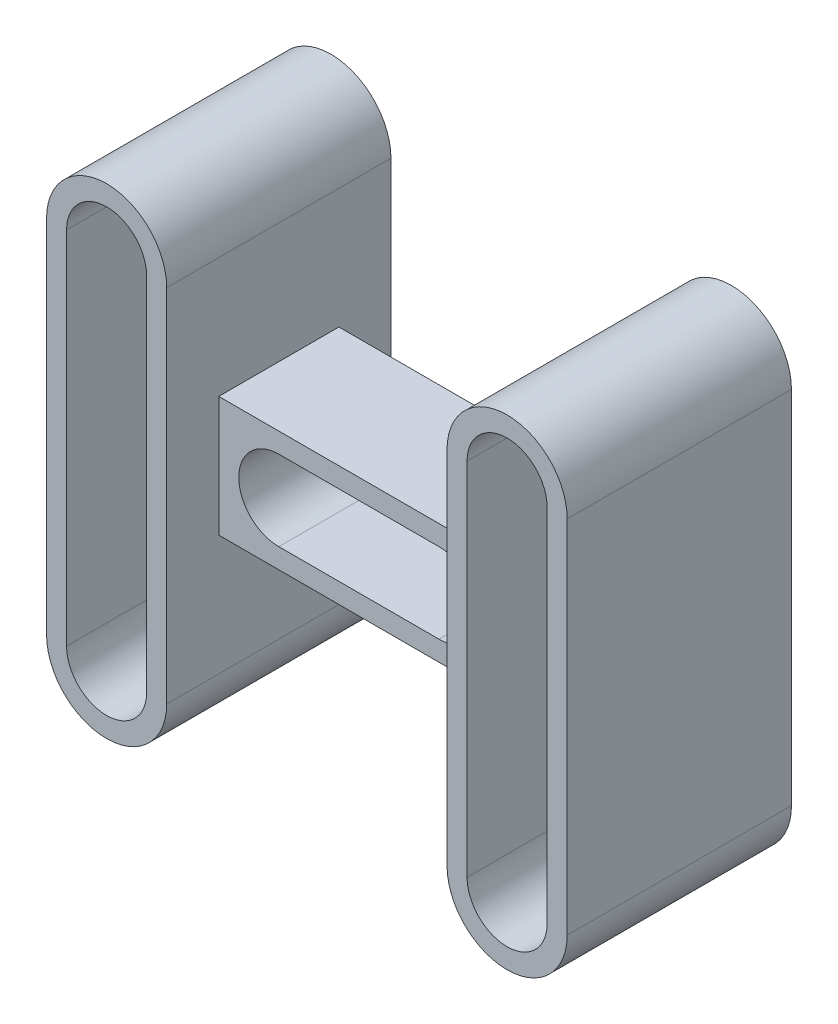
ISO-10303-21;
HEADER;
FILE_DESCRIPTION(('STEP AP214'),'2;1');
FILE_NAME('part.step','',(''),(''),'','','');
FILE_SCHEMA(('AUTOMOTIVE_DESIGN { 1 0 10303 214 1 1 1 1 }'));
ENDSEC;
DATA;
#1=APPLICATION_CONTEXT('core data for automotive mechanical design processes');
#2=APPLICATION_PROTOCOL_DEFINITION('international standard','automotive_design',2000,#1);
#3=PRODUCT_CONTEXT('',#1,'mechanical');
#4=PRODUCT('Part','Part','',(#3));
#5=PRODUCT_RELATED_PRODUCT_CATEGORY('part','',(#4));
#6=PRODUCT_DEFINITION_FORMATION('','',#4);
#7=PRODUCT_DEFINITION_CONTEXT('part definition',#1,'design');
#8=PRODUCT_DEFINITION('design','',#6,#7);
#9=PRODUCT_DEFINITION_SHAPE('','',#8);
#10=(LENGTH_UNIT() NAMED_UNIT(*) SI_UNIT(.MILLI.,.METRE.));
#11=(NAMED_UNIT(*) PLANE_ANGLE_UNIT() SI_UNIT($,.RADIAN.));
#12=(NAMED_UNIT(*) SI_UNIT($,.STERADIAN.) SOLID_ANGLE_UNIT());
#13=UNCERTAINTY_MEASURE_WITH_UNIT(LENGTH_MEASURE(1.E-05),#10,'distance_accuracy_value','');
#14=(GEOMETRIC_REPRESENTATION_CONTEXT(3) GLOBAL_UNCERTAINTY_ASSIGNED_CONTEXT((#13)) GLOBAL_UNIT_ASSIGNED_CONTEXT((#10,
#11,#12)) REPRESENTATION_CONTEXT('',''));
#15=CARTESIAN_POINT('',(0.,0.,0.));
#16=DIRECTION('',(0.,0.,1.));
#17=DIRECTION('',(1.,0.,0.));
#18=AXIS2_PLACEMENT_3D('',#15,#16,#17);
#19=CARTESIAN_POINT('',(35.,15.,15.));
#20=DIRECTION('',(0.,-1.,0.));
#21=DIRECTION('',(1.,0.,0.));
#22=AXIS2_PLACEMENT_3D('',#19,#20,#21);
#23=PLANE('',#22);
#24=DIRECTION('',(-1.,0.,0.));
#25=VECTOR('',#24,1.);
#26=CARTESIAN_POINT('',(35.,15.,-15.));
#27=LINE('',#26,#25);
#28=CARTESIAN_POINT('',(35.,15.,-15.));
#29=VERTEX_POINT('',#28);
#30=CARTESIAN_POINT('',(-35.,15.,-15.));
#31=VERTEX_POINT('',#30);
#32=EDGE_CURVE('E369',#29,#31,#27,.T.);
#33=ORIENTED_EDGE('',*,*,#32,.T.);
#34=DIRECTION('',(0.,0.,-1.));
#35=VECTOR('',#34,1.);
#36=CARTESIAN_POINT('',(-35.,15.,15.));
#37=LINE('',#36,#35);
#38=CARTESIAN_POINT('',(-35.,15.,15.));
#39=VERTEX_POINT('',#38);
#40=EDGE_CURVE('E381',#39,#31,#37,.T.);
#41=ORIENTED_EDGE('',*,*,#40,.F.);
#42=DIRECTION('',(-1.,0.,0.));
#43=VECTOR('',#42,1.);
#44=CARTESIAN_POINT('',(35.,15.,15.));
#45=LINE('',#44,#43);
#46=CARTESIAN_POINT('',(35.,15.,15.));
#47=VERTEX_POINT('',#46);
#48=EDGE_CURVE('E356',#47,#39,#45,.T.);
#49=ORIENTED_EDGE('',*,*,#48,.F.);
#50=DIRECTION('',(0.,0.,-1.));
#51=VECTOR('',#50,1.);
#52=CARTESIAN_POINT('',(35.,15.,15.));
#53=LINE('',#52,#51);
#54=EDGE_CURVE('E383',#47,#29,#53,.T.);
#55=ORIENTED_EDGE('',*,*,#54,.T.);
#56=EDGE_LOOP('',(#33,#41,#49,#55));
#57=FACE_BOUND('',#56,.T.);
#58=ADVANCED_FACE('F44',(#57),#23,.F.);
#59=CARTESIAN_POINT('',(-35.,-15.,15.));
#60=DIRECTION('',(0.,1.,0.));
#61=DIRECTION('',(0.,0.,1.));
#62=AXIS2_PLACEMENT_3D('',#59,#60,#61);
#63=PLANE('',#62);
#64=DIRECTION('',(1.,0.,0.));
#65=VECTOR('',#64,1.);
#66=CARTESIAN_POINT('',(-35.,-15.,-15.));
#67=LINE('',#66,#65);
#68=CARTESIAN_POINT('',(-35.,-15.,-15.));
#69=VERTEX_POINT('',#68);
#70=CARTESIAN_POINT('',(35.,-15.,-15.));
#71=VERTEX_POINT('',#70);
#72=EDGE_CURVE('E358',#69,#71,#67,.T.);
#73=ORIENTED_EDGE('',*,*,#72,.T.);
#74=DIRECTION('',(0.,0.,-1.));
#75=VECTOR('',#74,1.);
#76=CARTESIAN_POINT('',(35.,-15.,15.));
#77=LINE('',#76,#75);
#78=CARTESIAN_POINT('',(35.,-15.,15.));
#79=VERTEX_POINT('',#78);
#80=EDGE_CURVE('E368',#79,#71,#77,.T.);
#81=ORIENTED_EDGE('',*,*,#80,.F.);
#82=DIRECTION('',(1.,0.,0.));
#83=VECTOR('',#82,1.);
#84=CARTESIAN_POINT('',(-35.,-15.,15.));
#85=LINE('',#84,#83);
#86=CARTESIAN_POINT('',(-35.,-15.,15.));
#87=VERTEX_POINT('',#86);
#88=EDGE_CURVE('E365',#87,#79,#85,.T.);
#89=ORIENTED_EDGE('',*,*,#88,.F.);
#90=DIRECTION('',(0.,0.,-1.));
#91=VECTOR('',#90,1.);
#92=CARTESIAN_POINT('',(-35.,-15.,15.));
#93=LINE('',#92,#91);
#94=EDGE_CURVE('E378',#87,#69,#93,.T.);
#95=ORIENTED_EDGE('',*,*,#94,.T.);
#96=EDGE_LOOP('',(#73,#81,#89,#95));
#97=FACE_BOUND('',#96,.T.);
#98=ADVANCED_FACE('F423',(#97),#63,.F.);
#99=CARTESIAN_POINT('',(0.,0.,15.));
#100=DIRECTION('',(0.,0.,1.));
#101=DIRECTION('',(1.,0.,0.));
#102=AXIS2_PLACEMENT_3D('',#99,#100,#101);
#103=PLANE('',#102);
#104=CARTESIAN_POINT('',(-20.,0.,15.));
#105=DIRECTION('',(0.,0.,1.));
#106=DIRECTION('',(1.,0.,0.));
#107=AXIS2_PLACEMENT_3D('',#104,#105,#106);
#108=CIRCLE('',#107,10.);
#109=CARTESIAN_POINT('',(-20.,10.,15.));
#110=VERTEX_POINT('',#109);
#111=CARTESIAN_POINT('',(-20.,-10.,15.));
#112=VERTEX_POINT('',#111);
#113=EDGE_CURVE('E56',#110,#112,#108,.T.);
#114=ORIENTED_EDGE('',*,*,#113,.F.);
#115=DIRECTION('',(-1.,0.,0.));
#116=VECTOR('',#115,1.);
#117=CARTESIAN_POINT('',(-20.,10.,15.));
#118=LINE('',#117,#116);
#119=CARTESIAN_POINT('',(20.,10.,15.));
#120=VERTEX_POINT('',#119);
#121=EDGE_CURVE('E347',#120,#110,#118,.T.);
#122=ORIENTED_EDGE('',*,*,#121,.F.);
#123=CARTESIAN_POINT('',(20.,0.,15.));
#124=DIRECTION('',(0.,0.,1.));
#125=DIRECTION('',(1.,0.,0.));
#126=AXIS2_PLACEMENT_3D('',#123,#124,#125);
#127=CIRCLE('',#126,10.);
#128=CARTESIAN_POINT('',(20.,-10.,15.));
#129=VERTEX_POINT('',#128);
#130=EDGE_CURVE('E344',#129,#120,#127,.T.);
#131=ORIENTED_EDGE('',*,*,#130,.F.);
#132=DIRECTION('',(1.,0.,0.));
#133=VECTOR('',#132,1.);
#134=CARTESIAN_POINT('',(-20.,-10.,15.));
#135=LINE('',#134,#133);
#136=EDGE_CURVE('E342',#112,#129,#135,.T.);
#137=ORIENTED_EDGE('',*,*,#136,.F.);
#138=EDGE_LOOP('',(#114,#122,#131,#137));
#139=FACE_BOUND('',#138,.T.);
#140=DIRECTION('',(0.,1.,0.));
#141=VECTOR('',#140,1.);
#142=CARTESIAN_POINT('',(35.,-15.,15.));
#143=LINE('',#142,#141);
#144=EDGE_CURVE('E360',#79,#47,#143,.T.);
#145=ORIENTED_EDGE('',*,*,#144,.T.);
#146=ORIENTED_EDGE('',*,*,#48,.T.);
#147=DIRECTION('',(0.,-1.,0.));
#148=VECTOR('',#147,1.);
#149=CARTESIAN_POINT('',(-35.,15.,15.));
#150=LINE('',#149,#148);
#151=EDGE_CURVE('E362',#39,#87,#150,.T.);
#152=ORIENTED_EDGE('',*,*,#151,.T.);
#153=ORIENTED_EDGE('',*,*,#88,.T.);
#154=EDGE_LOOP('',(#145,#146,#152,#153));
#155=FACE_BOUND('',#154,.T.);
#156=ADVANCED_FACE('F408',(#139,#155),#103,.T.);
#157=CARTESIAN_POINT('',(0.,0.,-15.));
#158=DIRECTION('',(0.,0.,1.));
#159=DIRECTION('',(1.,0.,0.));
#160=AXIS2_PLACEMENT_3D('',#157,#158,#159);
#161=PLANE('',#160);
#162=DIRECTION('',(-1.,0.,0.));
#163=VECTOR('',#162,1.);
#164=CARTESIAN_POINT('',(0.,10.,-15.));
#165=LINE('',#164,#163);
#166=CARTESIAN_POINT('',(20.,10.,-15.));
#167=VERTEX_POINT('',#166);
#168=CARTESIAN_POINT('',(-20.,10.,-15.));
#169=VERTEX_POINT('',#168);
#170=EDGE_CURVE('E55',#167,#169,#165,.T.);
#171=ORIENTED_EDGE('',*,*,#170,.T.);
#172=CARTESIAN_POINT('',(-20.,0.,-15.));
#173=DIRECTION('',(0.,0.,1.));
#174=DIRECTION('',(1.,0.,0.));
#175=AXIS2_PLACEMENT_3D('',#172,#173,#174);
#176=CIRCLE('',#175,10.);
#177=CARTESIAN_POINT('',(-20.,-10.,-15.));
#178=VERTEX_POINT('',#177);
#179=EDGE_CURVE('E11',#169,#178,#176,.T.);
#180=ORIENTED_EDGE('',*,*,#179,.T.);
#181=DIRECTION('',(1.,0.,0.));
#182=VECTOR('',#181,1.);
#183=CARTESIAN_POINT('',(0.,-10.,-15.));
#184=LINE('',#183,#182);
#185=CARTESIAN_POINT('',(20.,-10.,-15.));
#186=VERTEX_POINT('',#185);
#187=EDGE_CURVE('E390',#178,#186,#184,.T.);
#188=ORIENTED_EDGE('',*,*,#187,.T.);
#189=CARTESIAN_POINT('',(20.,0.,-15.));
#190=DIRECTION('',(0.,0.,1.));
#191=DIRECTION('',(1.,0.,0.));
#192=AXIS2_PLACEMENT_3D('',#189,#190,#191);
#193=CIRCLE('',#192,10.);
#194=EDGE_CURVE('E388',#186,#167,#193,.T.);
#195=ORIENTED_EDGE('',*,*,#194,.T.);
#196=EDGE_LOOP('',(#171,#180,#188,#195));
#197=FACE_BOUND('',#196,.T.);
#198=DIRECTION('',(0.,1.,0.));
#199=VECTOR('',#198,1.);
#200=CARTESIAN_POINT('',(35.,0.,-15.));
#201=LINE('',#200,#199);
#202=EDGE_CURVE('E355',#71,#29,#201,.T.);
#203=ORIENTED_EDGE('',*,*,#202,.F.);
#204=ORIENTED_EDGE('',*,*,#72,.F.);
#205=DIRECTION('',(0.,-1.,0.));
#206=VECTOR('',#205,1.);
#207=CARTESIAN_POINT('',(-35.,15.,-15.));
#208=LINE('',#207,#206);
#209=EDGE_CURVE('E371',#31,#69,#208,.T.);
#210=ORIENTED_EDGE('',*,*,#209,.F.);
#211=ORIENTED_EDGE('',*,*,#32,.F.);
#212=EDGE_LOOP('',(#203,#204,#210,#211));
#213=FACE_BOUND('',#212,.T.);
#214=ADVANCED_FACE('F394',(#197,#213),#161,.F.);
#215=CARTESIAN_POINT('',(-20.,0.,-65.));
#216=DIRECTION('',(0.,0.,1.));
#217=DIRECTION('',(1.,0.,0.));
#218=AXIS2_PLACEMENT_3D('',#215,#216,#217);
#219=CYLINDRICAL_SURFACE('',#218,10.);
#220=DIRECTION('',(0.,0.,1.));
#221=VECTOR('',#220,1.);
#222=CARTESIAN_POINT('',(-20.,10.,-65.));
#223=LINE('',#222,#221);
#224=EDGE_CURVE('E348',#169,#110,#223,.T.);
#225=ORIENTED_EDGE('',*,*,#224,.T.);
#226=ORIENTED_EDGE('',*,*,#113,.T.);
#227=DIRECTION('',(0.,0.,1.));
#228=VECTOR('',#227,1.);
#229=CARTESIAN_POINT('',(-20.,-10.,-65.));
#230=LINE('',#229,#228);
#231=EDGE_CURVE('E349',#178,#112,#230,.T.);
#232=ORIENTED_EDGE('',*,*,#231,.F.);
#233=ORIENTED_EDGE('',*,*,#179,.F.);
#234=EDGE_LOOP('',(#225,#226,#232,#233));
#235=FACE_BOUND('',#234,.T.);
#236=ADVANCED_FACE('F409',(#235),#219,.F.);
#237=CARTESIAN_POINT('',(-20.,10.,-65.));
#238=DIRECTION('',(0.,1.,0.));
#239=DIRECTION('',(-1.,0.,0.));
#240=AXIS2_PLACEMENT_3D('',#237,#238,#239);
#241=PLANE('',#240);
#242=DIRECTION('',(0.,0.,1.));
#243=VECTOR('',#242,1.);
#244=CARTESIAN_POINT('',(20.,10.,-65.));
#245=LINE('',#244,#243);
#246=EDGE_CURVE('E351',#167,#120,#245,.T.);
#247=ORIENTED_EDGE('',*,*,#246,.T.);
#248=ORIENTED_EDGE('',*,*,#121,.T.);
#249=ORIENTED_EDGE('',*,*,#224,.F.);
#250=ORIENTED_EDGE('',*,*,#170,.F.);
#251=EDGE_LOOP('',(#247,#248,#249,#250));
#252=FACE_BOUND('',#251,.T.);
#253=ADVANCED_FACE('F396',(#252),#241,.F.);
#254=CARTESIAN_POINT('',(20.,0.,-65.));
#255=DIRECTION('',(0.,0.,1.));
#256=DIRECTION('',(1.,0.,0.));
#257=AXIS2_PLACEMENT_3D('',#254,#255,#256);
#258=CYLINDRICAL_SURFACE('',#257,10.);
#259=DIRECTION('',(0.,0.,1.));
#260=VECTOR('',#259,1.);
#261=CARTESIAN_POINT('',(20.,-10.,-65.));
#262=LINE('',#261,#260);
#263=EDGE_CURVE('E70',#186,#129,#262,.T.);
#264=ORIENTED_EDGE('',*,*,#263,.T.);
#265=ORIENTED_EDGE('',*,*,#130,.T.);
#266=ORIENTED_EDGE('',*,*,#246,.F.);
#267=ORIENTED_EDGE('',*,*,#194,.F.);
#268=EDGE_LOOP('',(#264,#265,#266,#267));
#269=FACE_BOUND('',#268,.T.);
#270=ADVANCED_FACE('F402',(#269),#258,.F.);
#271=CARTESIAN_POINT('',(-20.,-10.,-65.));
#272=DIRECTION('',(0.,-1.,0.));
#273=DIRECTION('',(1.,0.,0.));
#274=AXIS2_PLACEMENT_3D('',#271,#272,#273);
#275=PLANE('',#274);
#276=ORIENTED_EDGE('',*,*,#231,.T.);
#277=ORIENTED_EDGE('',*,*,#136,.T.);
#278=ORIENTED_EDGE('',*,*,#263,.F.);
#279=ORIENTED_EDGE('',*,*,#187,.F.);
#280=EDGE_LOOP('',(#276,#277,#278,#279));
#281=FACE_BOUND('',#280,.T.);
#282=ADVANCED_FACE('F406',(#281),#275,.F.);
#283=CARTESIAN_POINT('',(50.,45.,28.));
#284=DIRECTION('',(0.,0.,1.));
#285=DIRECTION('',(1.,0.,0.));
#286=AXIS2_PLACEMENT_3D('',#283,#284,#285);
#287=PLANE('',#286);
#288=DIRECTION('',(0.,-1.,0.));
#289=VECTOR('',#288,1.);
#290=CARTESIAN_POINT('',(35.,-15.,28.));
#291=LINE('',#290,#289);
#292=CARTESIAN_POINT('',(35.,45.,28.));
#293=VERTEX_POINT('',#292);
#294=CARTESIAN_POINT('',(35.,-45.,28.));
#295=VERTEX_POINT('',#294);
#296=EDGE_CURVE('E315',#293,#295,#291,.T.);
#297=ORIENTED_EDGE('',*,*,#296,.T.);
#298=CARTESIAN_POINT('',(50.,-45.,28.));
#299=DIRECTION('',(0.,0.,1.));
#300=DIRECTION('',(1.,0.,0.));
#301=AXIS2_PLACEMENT_3D('',#298,#299,#300);
#302=CIRCLE('',#301,15.);
#303=CARTESIAN_POINT('',(65.,-45.,28.));
#304=VERTEX_POINT('',#303);
#305=EDGE_CURVE('E314',#295,#304,#302,.T.);
#306=ORIENTED_EDGE('',*,*,#305,.T.);
#307=DIRECTION('',(0.,1.,0.));
#308=VECTOR('',#307,1.);
#309=CARTESIAN_POINT('',(65.,45.,28.));
#310=LINE('',#309,#308);
#311=CARTESIAN_POINT('',(65.,45.,28.));
#312=VERTEX_POINT('',#311);
#313=EDGE_CURVE('E320',#304,#312,#310,.T.);
#314=ORIENTED_EDGE('',*,*,#313,.T.);
#315=CARTESIAN_POINT('',(50.,45.,28.));
#316=DIRECTION('',(0.,0.,1.));
#317=DIRECTION('',(1.,0.,0.));
#318=AXIS2_PLACEMENT_3D('',#315,#316,#317);
#319=CIRCLE('',#318,15.);
#320=EDGE_CURVE('E317',#312,#293,#319,.T.);
#321=ORIENTED_EDGE('',*,*,#320,.T.);
#322=EDGE_LOOP('',(#297,#306,#314,#321));
#323=FACE_BOUND('',#322,.T.);
#324=DIRECTION('',(0.,-1.,0.));
#325=VECTOR('',#324,1.);
#326=CARTESIAN_POINT('',(40.,45.,28.));
#327=LINE('',#326,#325);
#328=CARTESIAN_POINT('',(40.,45.,28.));
#329=VERTEX_POINT('',#328);
#330=CARTESIAN_POINT('',(40.,-45.,28.));
#331=VERTEX_POINT('',#330);
#332=EDGE_CURVE('E281',#329,#331,#327,.T.);
#333=ORIENTED_EDGE('',*,*,#332,.F.);
#334=CARTESIAN_POINT('',(50.,45.,28.));
#335=DIRECTION('',(0.,0.,1.));
#336=DIRECTION('',(1.,0.,0.));
#337=AXIS2_PLACEMENT_3D('',#334,#335,#336);
#338=CIRCLE('',#337,10.);
#339=CARTESIAN_POINT('',(60.,45.,28.));
#340=VERTEX_POINT('',#339);
#341=EDGE_CURVE('E283',#340,#329,#338,.T.);
#342=ORIENTED_EDGE('',*,*,#341,.F.);
#343=DIRECTION('',(0.,1.,0.));
#344=VECTOR('',#343,1.);
#345=CARTESIAN_POINT('',(60.,45.,28.));
#346=LINE('',#345,#344);
#347=CARTESIAN_POINT('',(60.,-45.,28.));
#348=VERTEX_POINT('',#347);
#349=EDGE_CURVE('E286',#348,#340,#346,.T.);
#350=ORIENTED_EDGE('',*,*,#349,.F.);
#351=CARTESIAN_POINT('',(50.,-45.,28.));
#352=DIRECTION('',(0.,0.,1.));
#353=DIRECTION('',(1.,0.,0.));
#354=AXIS2_PLACEMENT_3D('',#351,#352,#353);
#355=CIRCLE('',#354,10.);
#356=EDGE_CURVE('E287',#331,#348,#355,.T.);
#357=ORIENTED_EDGE('',*,*,#356,.F.);
#358=EDGE_LOOP('',(#333,#342,#350,#357));
#359=FACE_BOUND('',#358,.T.);
#360=ADVANCED_FACE('F467',(#323,#359),#287,.T.);
#361=CARTESIAN_POINT('',(50.,45.,-28.));
#362=DIRECTION('',(0.,0.,1.));
#363=DIRECTION('',(1.,0.,0.));
#364=AXIS2_PLACEMENT_3D('',#361,#362,#363);
#365=PLANE('',#364);
#366=CARTESIAN_POINT('',(50.,-45.,-28.));
#367=DIRECTION('',(0.,0.,1.));
#368=DIRECTION('',(1.,0.,0.));
#369=AXIS2_PLACEMENT_3D('',#366,#367,#368);
#370=CIRCLE('',#369,15.);
#371=CARTESIAN_POINT('',(35.,-45.,-28.));
#372=VERTEX_POINT('',#371);
#373=CARTESIAN_POINT('',(65.,-45.,-28.));
#374=VERTEX_POINT('',#373);
#375=EDGE_CURVE('E313',#372,#374,#370,.T.);
#376=ORIENTED_EDGE('',*,*,#375,.F.);
#377=DIRECTION('',(0.,-1.,0.));
#378=VECTOR('',#377,1.);
#379=CARTESIAN_POINT('',(35.,0.,-28.));
#380=LINE('',#379,#378);
#381=CARTESIAN_POINT('',(35.,45.,-28.));
#382=VERTEX_POINT('',#381);
#383=EDGE_CURVE('E312',#382,#372,#380,.T.);
#384=ORIENTED_EDGE('',*,*,#383,.F.);
#385=CARTESIAN_POINT('',(50.,45.,-28.));
#386=DIRECTION('',(0.,0.,1.));
#387=DIRECTION('',(1.,0.,0.));
#388=AXIS2_PLACEMENT_3D('',#385,#386,#387);
#389=CIRCLE('',#388,15.);
#390=CARTESIAN_POINT('',(65.,45.,-28.));
#391=VERTEX_POINT('',#390);
#392=EDGE_CURVE('E326',#391,#382,#389,.T.);
#393=ORIENTED_EDGE('',*,*,#392,.F.);
#394=DIRECTION('',(0.,1.,0.));
#395=VECTOR('',#394,1.);
#396=CARTESIAN_POINT('',(65.,45.,-28.));
#397=LINE('',#396,#395);
#398=EDGE_CURVE('E322',#374,#391,#397,.T.);
#399=ORIENTED_EDGE('',*,*,#398,.F.);
#400=EDGE_LOOP('',(#376,#384,#393,#399));
#401=FACE_BOUND('',#400,.T.);
#402=CARTESIAN_POINT('',(50.,45.,-28.));
#403=DIRECTION('',(0.,0.,1.));
#404=DIRECTION('',(1.,0.,0.));
#405=AXIS2_PLACEMENT_3D('',#402,#403,#404);
#406=CIRCLE('',#405,10.);
#407=CARTESIAN_POINT('',(60.,45.,-28.));
#408=VERTEX_POINT('',#407);
#409=CARTESIAN_POINT('',(40.,45.,-28.));
#410=VERTEX_POINT('',#409);
#411=EDGE_CURVE('E278',#408,#410,#406,.T.);
#412=ORIENTED_EDGE('',*,*,#411,.T.);
#413=DIRECTION('',(0.,-1.,0.));
#414=VECTOR('',#413,1.);
#415=CARTESIAN_POINT('',(40.,45.,-28.));
#416=LINE('',#415,#414);
#417=CARTESIAN_POINT('',(40.,-45.,-28.));
#418=VERTEX_POINT('',#417);
#419=EDGE_CURVE('E294',#410,#418,#416,.T.);
#420=ORIENTED_EDGE('',*,*,#419,.T.);
#421=CARTESIAN_POINT('',(50.,-45.,-28.));
#422=DIRECTION('',(0.,0.,1.));
#423=DIRECTION('',(1.,0.,0.));
#424=AXIS2_PLACEMENT_3D('',#421,#422,#423);
#425=CIRCLE('',#424,10.);
#426=CARTESIAN_POINT('',(60.,-45.,-28.));
#427=VERTEX_POINT('',#426);
#428=EDGE_CURVE('E300',#418,#427,#425,.T.);
#429=ORIENTED_EDGE('',*,*,#428,.T.);
#430=DIRECTION('',(0.,1.,0.));
#431=VECTOR('',#430,1.);
#432=CARTESIAN_POINT('',(60.,45.,-28.));
#433=LINE('',#432,#431);
#434=EDGE_CURVE('E284',#427,#408,#433,.T.);
#435=ORIENTED_EDGE('',*,*,#434,.T.);
#436=EDGE_LOOP('',(#412,#420,#429,#435));
#437=FACE_BOUND('',#436,.T.);
#438=ADVANCED_FACE('F460',(#401,#437),#365,.F.);
#439=CARTESIAN_POINT('',(50.,-45.,28.));
#440=DIRECTION('',(0.,0.,-1.));
#441=DIRECTION('',(-1.,0.,0.));
#442=AXIS2_PLACEMENT_3D('',#439,#440,#441);
#443=CYLINDRICAL_SURFACE('',#442,15.);
#444=ORIENTED_EDGE('',*,*,#375,.T.);
#445=DIRECTION('',(0.,0.,-1.));
#446=VECTOR('',#445,1.);
#447=CARTESIAN_POINT('',(65.,-45.,28.));
#448=LINE('',#447,#446);
#449=EDGE_CURVE('E331',#304,#374,#448,.T.);
#450=ORIENTED_EDGE('',*,*,#449,.F.);
#451=ORIENTED_EDGE('',*,*,#305,.F.);
#452=DIRECTION('',(0.,0.,-1.));
#453=VECTOR('',#452,1.);
#454=CARTESIAN_POINT('',(35.,-45.,28.));
#455=LINE('',#454,#453);
#456=EDGE_CURVE('E340',#295,#372,#455,.T.);
#457=ORIENTED_EDGE('',*,*,#456,.T.);
#458=EDGE_LOOP('',(#444,#450,#451,#457));
#459=FACE_BOUND('',#458,.T.);
#460=ADVANCED_FACE('F451',(#459),#443,.T.);
#461=CARTESIAN_POINT('',(65.,45.,28.));
#462=DIRECTION('',(-1.,0.,0.));
#463=DIRECTION('',(0.,-1.,0.));
#464=AXIS2_PLACEMENT_3D('',#461,#462,#463);
#465=PLANE('',#464);
#466=ORIENTED_EDGE('',*,*,#398,.T.);
#467=DIRECTION('',(0.,0.,-1.));
#468=VECTOR('',#467,1.);
#469=CARTESIAN_POINT('',(65.,45.,28.));
#470=LINE('',#469,#468);
#471=EDGE_CURVE('E332',#312,#391,#470,.T.);
#472=ORIENTED_EDGE('',*,*,#471,.F.);
#473=ORIENTED_EDGE('',*,*,#313,.F.);
#474=ORIENTED_EDGE('',*,*,#449,.T.);
#475=EDGE_LOOP('',(#466,#472,#473,#474));
#476=FACE_BOUND('',#475,.T.);
#477=ADVANCED_FACE('F463',(#476),#465,.F.);
#478=CARTESIAN_POINT('',(50.,45.,28.));
#479=DIRECTION('',(0.,0.,-1.));
#480=DIRECTION('',(-1.,0.,0.));
#481=AXIS2_PLACEMENT_3D('',#478,#479,#480);
#482=CYLINDRICAL_SURFACE('',#481,15.);
#483=ORIENTED_EDGE('',*,*,#392,.T.);
#484=DIRECTION('',(0.,0.,-1.));
#485=VECTOR('',#484,1.);
#486=CARTESIAN_POINT('',(35.,45.,28.));
#487=LINE('',#486,#485);
#488=EDGE_CURVE('E325',#293,#382,#487,.T.);
#489=ORIENTED_EDGE('',*,*,#488,.F.);
#490=ORIENTED_EDGE('',*,*,#320,.F.);
#491=ORIENTED_EDGE('',*,*,#471,.T.);
#492=EDGE_LOOP('',(#483,#489,#490,#491));
#493=FACE_BOUND('',#492,.T.);
#494=ADVANCED_FACE('F441',(#493),#482,.T.);
#495=CARTESIAN_POINT('',(35.,0.,28.));
#496=DIRECTION('',(1.,0.,0.));
#497=DIRECTION('',(0.,0.,-1.));
#498=AXIS2_PLACEMENT_3D('',#495,#496,#497);
#499=PLANE('',#498);
#500=ORIENTED_EDGE('',*,*,#144,.F.);
#501=ORIENTED_EDGE('',*,*,#80,.T.);
#502=ORIENTED_EDGE('',*,*,#202,.T.);
#503=ORIENTED_EDGE('',*,*,#54,.F.);
#504=EDGE_LOOP('',(#500,#501,#502,#503));
#505=FACE_BOUND('',#504,.T.);
#506=ORIENTED_EDGE('',*,*,#383,.T.);
#507=ORIENTED_EDGE('',*,*,#456,.F.);
#508=ORIENTED_EDGE('',*,*,#296,.F.);
#509=ORIENTED_EDGE('',*,*,#488,.T.);
#510=EDGE_LOOP('',(#506,#507,#508,#509));
#511=FACE_BOUND('',#510,.T.);
#512=ADVANCED_FACE('F439',(#505,#511),#499,.F.);
#513=CARTESIAN_POINT('',(50.,45.,28.));
#514=DIRECTION('',(0.,0.,-1.));
#515=DIRECTION('',(-1.,0.,0.));
#516=AXIS2_PLACEMENT_3D('',#513,#514,#515);
#517=CYLINDRICAL_SURFACE('',#516,10.);
#518=ORIENTED_EDGE('',*,*,#411,.F.);
#519=DIRECTION('',(0.,0.,-1.));
#520=VECTOR('',#519,1.);
#521=CARTESIAN_POINT('',(60.,45.,28.));
#522=LINE('',#521,#520);
#523=EDGE_CURVE('E292',#340,#408,#522,.T.);
#524=ORIENTED_EDGE('',*,*,#523,.F.);
#525=ORIENTED_EDGE('',*,*,#341,.T.);
#526=DIRECTION('',(0.,0.,-1.));
#527=VECTOR('',#526,1.);
#528=CARTESIAN_POINT('',(40.,45.,28.));
#529=LINE('',#528,#527);
#530=EDGE_CURVE('E306',#329,#410,#529,.T.);
#531=ORIENTED_EDGE('',*,*,#530,.T.);
#532=EDGE_LOOP('',(#518,#524,#525,#531));
#533=FACE_BOUND('',#532,.T.);
#534=ADVANCED_FACE('F444',(#533),#517,.F.);
#535=CARTESIAN_POINT('',(40.,45.,28.));
#536=DIRECTION('',(1.,0.,0.));
#537=DIRECTION('',(0.,1.,0.));
#538=AXIS2_PLACEMENT_3D('',#535,#536,#537);
#539=PLANE('',#538);
#540=ORIENTED_EDGE('',*,*,#419,.F.);
#541=ORIENTED_EDGE('',*,*,#530,.F.);
#542=ORIENTED_EDGE('',*,*,#332,.T.);
#543=DIRECTION('',(0.,0.,-1.));
#544=VECTOR('',#543,1.);
#545=CARTESIAN_POINT('',(40.,-45.,28.));
#546=LINE('',#545,#544);
#547=EDGE_CURVE('E308',#331,#418,#546,.T.);
#548=ORIENTED_EDGE('',*,*,#547,.T.);
#549=EDGE_LOOP('',(#540,#541,#542,#548));
#550=FACE_BOUND('',#549,.T.);
#551=ADVANCED_FACE('F480',(#550),#539,.T.);
#552=CARTESIAN_POINT('',(50.,-45.,28.));
#553=DIRECTION('',(0.,0.,-1.));
#554=DIRECTION('',(-1.,0.,0.));
#555=AXIS2_PLACEMENT_3D('',#552,#553,#554);
#556=CYLINDRICAL_SURFACE('',#555,10.);
#557=ORIENTED_EDGE('',*,*,#428,.F.);
#558=ORIENTED_EDGE('',*,*,#547,.F.);
#559=ORIENTED_EDGE('',*,*,#356,.T.);
#560=DIRECTION('',(0.,0.,-1.));
#561=VECTOR('',#560,1.);
#562=CARTESIAN_POINT('',(60.,-45.,28.));
#563=LINE('',#562,#561);
#564=EDGE_CURVE('E301',#348,#427,#563,.T.);
#565=ORIENTED_EDGE('',*,*,#564,.T.);
#566=EDGE_LOOP('',(#557,#558,#559,#565));
#567=FACE_BOUND('',#566,.T.);
#568=ADVANCED_FACE('F477',(#567),#556,.F.);
#569=CARTESIAN_POINT('',(60.,45.,28.));
#570=DIRECTION('',(-1.,0.,0.));
#571=DIRECTION('',(0.,-1.,0.));
#572=AXIS2_PLACEMENT_3D('',#569,#570,#571);
#573=PLANE('',#572);
#574=ORIENTED_EDGE('',*,*,#434,.F.);
#575=ORIENTED_EDGE('',*,*,#564,.F.);
#576=ORIENTED_EDGE('',*,*,#349,.T.);
#577=ORIENTED_EDGE('',*,*,#523,.T.);
#578=EDGE_LOOP('',(#574,#575,#576,#577));
#579=FACE_BOUND('',#578,.T.);
#580=ADVANCED_FACE('F484',(#579),#573,.T.);
#581=CARTESIAN_POINT('',(-50.,45.,28.));
#582=DIRECTION('',(0.,0.,-1.));
#583=DIRECTION('',(-1.,0.,0.));
#584=AXIS2_PLACEMENT_3D('',#581,#582,#583);
#585=CYLINDRICAL_SURFACE('',#584,15.);
#586=CARTESIAN_POINT('',(-50.,45.,-28.));
#587=DIRECTION('',(0.,0.,-1.));
#588=DIRECTION('',(-1.,0.,0.));
#589=AXIS2_PLACEMENT_3D('',#586,#587,#588);
#590=CIRCLE('',#589,15.);
#591=CARTESIAN_POINT('',(-65.,45.,-28.));
#592=VERTEX_POINT('',#591);
#593=CARTESIAN_POINT('',(-35.,45.,-28.));
#594=VERTEX_POINT('',#593);
#595=EDGE_CURVE('E216',#592,#594,#590,.T.);
#596=ORIENTED_EDGE('',*,*,#595,.F.);
#597=DIRECTION('',(0.,0.,-1.));
#598=VECTOR('',#597,1.);
#599=CARTESIAN_POINT('',(-65.,45.,28.));
#600=LINE('',#599,#598);
#601=CARTESIAN_POINT('',(-65.,45.,28.));
#602=VERTEX_POINT('',#601);
#603=EDGE_CURVE('E274',#602,#592,#600,.T.);
#604=ORIENTED_EDGE('',*,*,#603,.F.);
#605=CARTESIAN_POINT('',(-50.,45.,28.));
#606=DIRECTION('',(0.,0.,-1.));
#607=DIRECTION('',(-1.,0.,0.));
#608=AXIS2_PLACEMENT_3D('',#605,#606,#607);
#609=CIRCLE('',#608,15.);
#610=CARTESIAN_POINT('',(-35.,45.,28.));
#611=VERTEX_POINT('',#610);
#612=EDGE_CURVE('E253',#602,#611,#609,.T.);
#613=ORIENTED_EDGE('',*,*,#612,.T.);
#614=DIRECTION('',(0.,0.,-1.));
#615=VECTOR('',#614,1.);
#616=CARTESIAN_POINT('',(-35.,45.,28.));
#617=LINE('',#616,#615);
#618=EDGE_CURVE('E280',#611,#594,#617,.T.);
#619=ORIENTED_EDGE('',*,*,#618,.T.);
#620=EDGE_LOOP('',(#596,#604,#613,#619));
#621=FACE_BOUND('',#620,.T.);
#622=ADVANCED_FACE('F490',(#621),#585,.T.);
#623=CARTESIAN_POINT('',(-65.,45.,28.));
#624=DIRECTION('',(-1.,0.,0.));
#625=DIRECTION('',(0.,-1.,0.));
#626=AXIS2_PLACEMENT_3D('',#623,#624,#625);
#627=PLANE('',#626);
#628=DIRECTION('',(0.,1.,0.));
#629=VECTOR('',#628,1.);
#630=CARTESIAN_POINT('',(-65.,45.,-28.));
#631=LINE('',#630,#629);
#632=CARTESIAN_POINT('',(-65.,-45.,-28.));
#633=VERTEX_POINT('',#632);
#634=EDGE_CURVE('E262',#633,#592,#631,.T.);
#635=ORIENTED_EDGE('',*,*,#634,.F.);
#636=DIRECTION('',(0.,0.,-1.));
#637=VECTOR('',#636,1.);
#638=CARTESIAN_POINT('',(-65.,-45.,28.));
#639=LINE('',#638,#637);
#640=CARTESIAN_POINT('',(-65.,-45.,28.));
#641=VERTEX_POINT('',#640);
#642=EDGE_CURVE('E272',#641,#633,#639,.T.);
#643=ORIENTED_EDGE('',*,*,#642,.F.);
#644=DIRECTION('',(0.,1.,0.));
#645=VECTOR('',#644,1.);
#646=CARTESIAN_POINT('',(-65.,45.,28.));
#647=LINE('',#646,#645);
#648=EDGE_CURVE('E254',#641,#602,#647,.T.);
#649=ORIENTED_EDGE('',*,*,#648,.T.);
#650=ORIENTED_EDGE('',*,*,#603,.T.);
#651=EDGE_LOOP('',(#635,#643,#649,#650));
#652=FACE_BOUND('',#651,.T.);
#653=ADVANCED_FACE('F492',(#652),#627,.T.);
#654=CARTESIAN_POINT('',(-50.,-45.,28.));
#655=DIRECTION('',(0.,0.,-1.));
#656=DIRECTION('',(-1.,0.,0.));
#657=AXIS2_PLACEMENT_3D('',#654,#655,#656);
#658=CYLINDRICAL_SURFACE('',#657,15.);
#659=CARTESIAN_POINT('',(-50.,-45.,-28.));
#660=DIRECTION('',(0.,0.,-1.));
#661=DIRECTION('',(-1.,0.,0.));
#662=AXIS2_PLACEMENT_3D('',#659,#660,#661);
#663=CIRCLE('',#662,15.);
#664=CARTESIAN_POINT('',(-35.,-45.,-28.));
#665=VERTEX_POINT('',#664);
#666=EDGE_CURVE('E270',#665,#633,#663,.T.);
#667=ORIENTED_EDGE('',*,*,#666,.F.);
#668=DIRECTION('',(0.,0.,-1.));
#669=VECTOR('',#668,1.);
#670=CARTESIAN_POINT('',(-35.,-45.,28.));
#671=LINE('',#670,#669);
#672=CARTESIAN_POINT('',(-35.,-45.,28.));
#673=VERTEX_POINT('',#672);
#674=EDGE_CURVE('E261',#673,#665,#671,.T.);
#675=ORIENTED_EDGE('',*,*,#674,.F.);
#676=CARTESIAN_POINT('',(-50.,-45.,28.));
#677=DIRECTION('',(0.,0.,-1.));
#678=DIRECTION('',(-1.,0.,0.));
#679=AXIS2_PLACEMENT_3D('',#676,#677,#678);
#680=CIRCLE('',#679,15.);
#681=EDGE_CURVE('E256',#673,#641,#680,.T.);
#682=ORIENTED_EDGE('',*,*,#681,.T.);
#683=ORIENTED_EDGE('',*,*,#642,.T.);
#684=EDGE_LOOP('',(#667,#675,#682,#683));
#685=FACE_BOUND('',#684,.T.);
#686=ADVANCED_FACE('F572',(#685),#658,.T.);
#687=CARTESIAN_POINT('',(-35.,-45.,28.));
#688=DIRECTION('',(1.,0.,0.));
#689=DIRECTION('',(0.,0.,-1.));
#690=AXIS2_PLACEMENT_3D('',#687,#688,#689);
#691=PLANE('',#690);
#692=ORIENTED_EDGE('',*,*,#94,.F.);
#693=ORIENTED_EDGE('',*,*,#151,.F.);
#694=ORIENTED_EDGE('',*,*,#40,.T.);
#695=ORIENTED_EDGE('',*,*,#209,.T.);
#696=EDGE_LOOP('',(#692,#693,#694,#695));
#697=FACE_BOUND('',#696,.T.);
#698=DIRECTION('',(0.,-1.,0.));
#699=VECTOR('',#698,1.);
#700=CARTESIAN_POINT('',(-35.,-45.,-28.));
#701=LINE('',#700,#699);
#702=EDGE_CURVE('E252',#594,#665,#701,.T.);
#703=ORIENTED_EDGE('',*,*,#702,.F.);
#704=ORIENTED_EDGE('',*,*,#618,.F.);
#705=DIRECTION('',(0.,-1.,0.));
#706=VECTOR('',#705,1.);
#707=CARTESIAN_POINT('',(-35.,-15.,28.));
#708=LINE('',#707,#706);
#709=EDGE_CURVE('E246',#611,#673,#708,.T.);
#710=ORIENTED_EDGE('',*,*,#709,.T.);
#711=ORIENTED_EDGE('',*,*,#674,.T.);
#712=EDGE_LOOP('',(#703,#704,#710,#711));
#713=FACE_BOUND('',#712,.T.);
#714=ADVANCED_FACE('F432',(#697,#713),#691,.T.);
#715=CARTESIAN_POINT('',(-50.,45.,28.));
#716=DIRECTION('',(0.,0.,1.));
#717=DIRECTION('',(-1.,0.,0.));
#718=AXIS2_PLACEMENT_3D('',#715,#716,#717);
#719=PLANE('',#718);
#720=CARTESIAN_POINT('',(-50.,45.,28.));
#721=DIRECTION('',(0.,0.,-1.));
#722=DIRECTION('',(-1.,0.,0.));
#723=AXIS2_PLACEMENT_3D('',#720,#721,#722);
#724=CIRCLE('',#723,10.);
#725=CARTESIAN_POINT('',(-60.,45.,28.));
#726=VERTEX_POINT('',#725);
#727=CARTESIAN_POINT('',(-40.,45.,28.));
#728=VERTEX_POINT('',#727);
#729=EDGE_CURVE('E219',#726,#728,#724,.T.);
#730=ORIENTED_EDGE('',*,*,#729,.T.);
#731=DIRECTION('',(0.,-1.,0.));
#732=VECTOR('',#731,1.);
#733=CARTESIAN_POINT('',(-40.,45.,28.));
#734=LINE('',#733,#732);
#735=CARTESIAN_POINT('',(-40.,-45.,28.));
#736=VERTEX_POINT('',#735);
#737=EDGE_CURVE('E234',#728,#736,#734,.T.);
#738=ORIENTED_EDGE('',*,*,#737,.T.);
#739=CARTESIAN_POINT('',(-50.,-45.,28.));
#740=DIRECTION('',(0.,0.,-1.));
#741=DIRECTION('',(-1.,0.,0.));
#742=AXIS2_PLACEMENT_3D('',#739,#740,#741);
#743=CIRCLE('',#742,10.);
#744=CARTESIAN_POINT('',(-60.,-45.,28.));
#745=VERTEX_POINT('',#744);
#746=EDGE_CURVE('E232',#736,#745,#743,.T.);
#747=ORIENTED_EDGE('',*,*,#746,.T.);
#748=DIRECTION('',(0.,1.,0.));
#749=VECTOR('',#748,1.);
#750=CARTESIAN_POINT('',(-60.,45.,28.));
#751=LINE('',#750,#749);
#752=EDGE_CURVE('E209',#745,#726,#751,.T.);
#753=ORIENTED_EDGE('',*,*,#752,.T.);
#754=EDGE_LOOP('',(#730,#738,#747,#753));
#755=FACE_BOUND('',#754,.T.);
#756=ORIENTED_EDGE('',*,*,#709,.F.);
#757=ORIENTED_EDGE('',*,*,#612,.F.);
#758=ORIENTED_EDGE('',*,*,#648,.F.);
#759=ORIENTED_EDGE('',*,*,#681,.F.);
#760=EDGE_LOOP('',(#756,#757,#758,#759));
#761=FACE_BOUND('',#760,.T.);
#762=ADVANCED_FACE('F229',(#755,#761),#719,.T.);
#763=CARTESIAN_POINT('',(-50.,45.,-28.));
#764=DIRECTION('',(0.,0.,1.));
#765=DIRECTION('',(-1.,0.,0.));
#766=AXIS2_PLACEMENT_3D('',#763,#764,#765);
#767=PLANE('',#766);
#768=DIRECTION('',(0.,-1.,0.));
#769=VECTOR('',#768,1.);
#770=CARTESIAN_POINT('',(-40.,45.,-28.));
#771=LINE('',#770,#769);
#772=CARTESIAN_POINT('',(-40.,45.,-28.));
#773=VERTEX_POINT('',#772);
#774=CARTESIAN_POINT('',(-40.,-45.,-28.));
#775=VERTEX_POINT('',#774);
#776=EDGE_CURVE('E230',#773,#775,#771,.T.);
#777=ORIENTED_EDGE('',*,*,#776,.F.);
#778=CARTESIAN_POINT('',(-50.,45.,-28.));
#779=DIRECTION('',(0.,0.,-1.));
#780=DIRECTION('',(-1.,0.,0.));
#781=AXIS2_PLACEMENT_3D('',#778,#779,#780);
#782=CIRCLE('',#781,10.);
#783=CARTESIAN_POINT('',(-60.,45.,-28.));
#784=VERTEX_POINT('',#783);
#785=EDGE_CURVE('E240',#784,#773,#782,.T.);
#786=ORIENTED_EDGE('',*,*,#785,.F.);
#787=DIRECTION('',(0.,1.,0.));
#788=VECTOR('',#787,1.);
#789=CARTESIAN_POINT('',(-60.,45.,-28.));
#790=LINE('',#789,#788);
#791=CARTESIAN_POINT('',(-60.,-45.,-28.));
#792=VERTEX_POINT('',#791);
#793=EDGE_CURVE('E213',#792,#784,#790,.T.);
#794=ORIENTED_EDGE('',*,*,#793,.F.);
#795=CARTESIAN_POINT('',(-50.,-45.,-28.));
#796=DIRECTION('',(0.,0.,-1.));
#797=DIRECTION('',(-1.,0.,0.));
#798=AXIS2_PLACEMENT_3D('',#795,#796,#797);
#799=CIRCLE('',#798,10.);
#800=EDGE_CURVE('E238',#775,#792,#799,.T.);
#801=ORIENTED_EDGE('',*,*,#800,.F.);
#802=EDGE_LOOP('',(#777,#786,#794,#801));
#803=FACE_BOUND('',#802,.T.);
#804=ORIENTED_EDGE('',*,*,#595,.T.);
#805=ORIENTED_EDGE('',*,*,#702,.T.);
#806=ORIENTED_EDGE('',*,*,#666,.T.);
#807=ORIENTED_EDGE('',*,*,#634,.T.);
#808=EDGE_LOOP('',(#804,#805,#806,#807));
#809=FACE_BOUND('',#808,.T.);
#810=ADVANCED_FACE('F599',(#803,#809),#767,.F.);
#811=CARTESIAN_POINT('',(-50.,45.,28.));
#812=DIRECTION('',(0.,0.,-1.));
#813=DIRECTION('',(-1.,0.,0.));
#814=AXIS2_PLACEMENT_3D('',#811,#812,#813);
#815=CYLINDRICAL_SURFACE('',#814,10.);
#816=ORIENTED_EDGE('',*,*,#785,.T.);
#817=DIRECTION('',(0.,0.,-1.));
#818=VECTOR('',#817,1.);
#819=CARTESIAN_POINT('',(-40.,45.,28.));
#820=LINE('',#819,#818);
#821=EDGE_CURVE('E224',#728,#773,#820,.T.);
#822=ORIENTED_EDGE('',*,*,#821,.F.);
#823=ORIENTED_EDGE('',*,*,#729,.F.);
#824=DIRECTION('',(0.,0.,-1.));
#825=VECTOR('',#824,1.);
#826=CARTESIAN_POINT('',(-60.,45.,28.));
#827=LINE('',#826,#825);
#828=EDGE_CURVE('E206',#726,#784,#827,.T.);
#829=ORIENTED_EDGE('',*,*,#828,.T.);
#830=EDGE_LOOP('',(#816,#822,#823,#829));
#831=FACE_BOUND('',#830,.T.);
#832=ADVANCED_FACE('F222',(#831),#815,.F.);
#833=CARTESIAN_POINT('',(-60.,45.,28.));
#834=DIRECTION('',(-1.,0.,0.));
#835=DIRECTION('',(0.,-1.,0.));
#836=AXIS2_PLACEMENT_3D('',#833,#834,#835);
#837=PLANE('',#836);
#838=ORIENTED_EDGE('',*,*,#793,.T.);
#839=ORIENTED_EDGE('',*,*,#828,.F.);
#840=ORIENTED_EDGE('',*,*,#752,.F.);
#841=DIRECTION('',(0.,0.,-1.));
#842=VECTOR('',#841,1.);
#843=CARTESIAN_POINT('',(-60.,-45.,28.));
#844=LINE('',#843,#842);
#845=EDGE_CURVE('E220',#745,#792,#844,.T.);
#846=ORIENTED_EDGE('',*,*,#845,.T.);
#847=EDGE_LOOP('',(#838,#839,#840,#846));
#848=FACE_BOUND('',#847,.T.);
#849=ADVANCED_FACE('F208',(#848),#837,.F.);
#850=CARTESIAN_POINT('',(-50.,-45.,28.));
#851=DIRECTION('',(0.,0.,-1.));
#852=DIRECTION('',(-1.,0.,0.));
#853=AXIS2_PLACEMENT_3D('',#850,#851,#852);
#854=CYLINDRICAL_SURFACE('',#853,10.);
#855=ORIENTED_EDGE('',*,*,#800,.T.);
#856=ORIENTED_EDGE('',*,*,#845,.F.);
#857=ORIENTED_EDGE('',*,*,#746,.F.);
#858=DIRECTION('',(0.,0.,-1.));
#859=VECTOR('',#858,1.);
#860=CARTESIAN_POINT('',(-40.,-45.,28.));
#861=LINE('',#860,#859);
#862=EDGE_CURVE('E247',#736,#775,#861,.T.);
#863=ORIENTED_EDGE('',*,*,#862,.T.);
#864=EDGE_LOOP('',(#855,#856,#857,#863));
#865=FACE_BOUND('',#864,.T.);
#866=ADVANCED_FACE('F628',(#865),#854,.F.);
#867=CARTESIAN_POINT('',(-40.,45.,28.));
#868=DIRECTION('',(1.,0.,0.));
#869=DIRECTION('',(0.,1.,0.));
#870=AXIS2_PLACEMENT_3D('',#867,#868,#869);
#871=PLANE('',#870);
#872=ORIENTED_EDGE('',*,*,#776,.T.);
#873=ORIENTED_EDGE('',*,*,#862,.F.);
#874=ORIENTED_EDGE('',*,*,#737,.F.);
#875=ORIENTED_EDGE('',*,*,#821,.T.);
#876=EDGE_LOOP('',(#872,#873,#874,#875));
#877=FACE_BOUND('',#876,.T.);
#878=ADVANCED_FACE('F633',(#877),#871,.F.);
#879=CLOSED_SHELL('',(#58,#98,#156,#214,#236,#253,#270,#282,#360,#438,#460,#477,#494,#512,#534,
#551,#568,#580,#622,#653,#686,#714,#762,#810,#832,#849,#866,#878));
#880=MANIFOLD_SOLID_BREP('B2',#879);
#881=ADVANCED_BREP_SHAPE_REPRESENTATION('',(#18,#880),#14);
#882=SHAPE_DEFINITION_REPRESENTATION(#9,#881);
ENDSEC;
END-ISO-10303-21;
